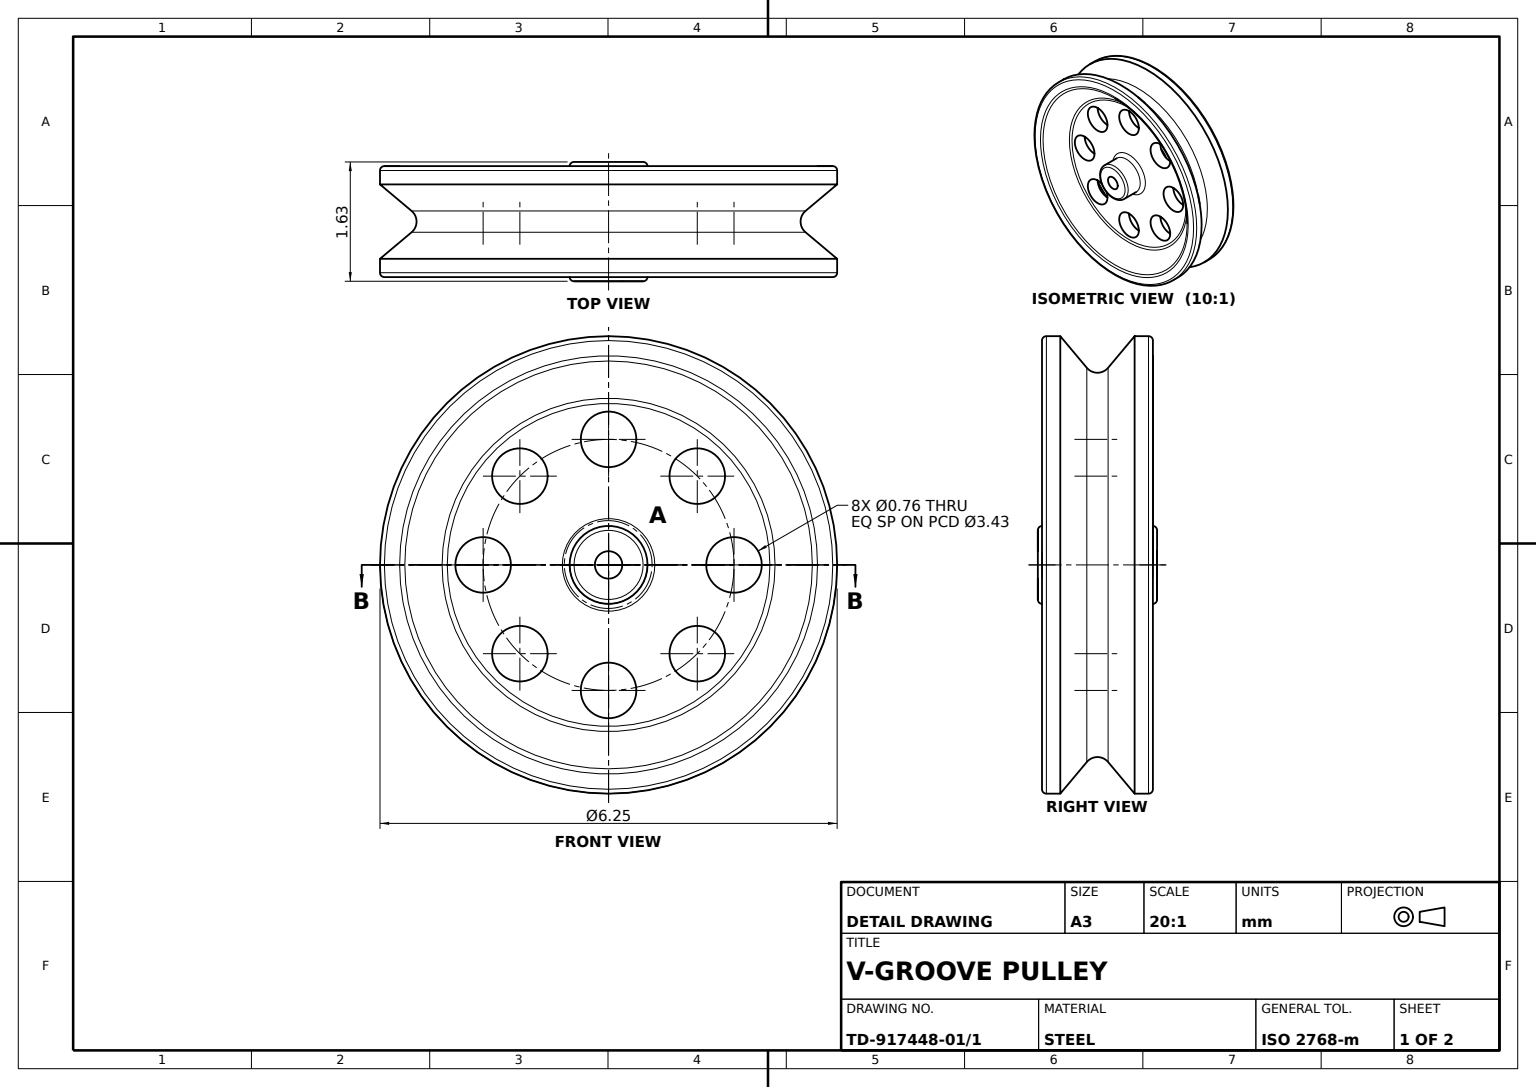
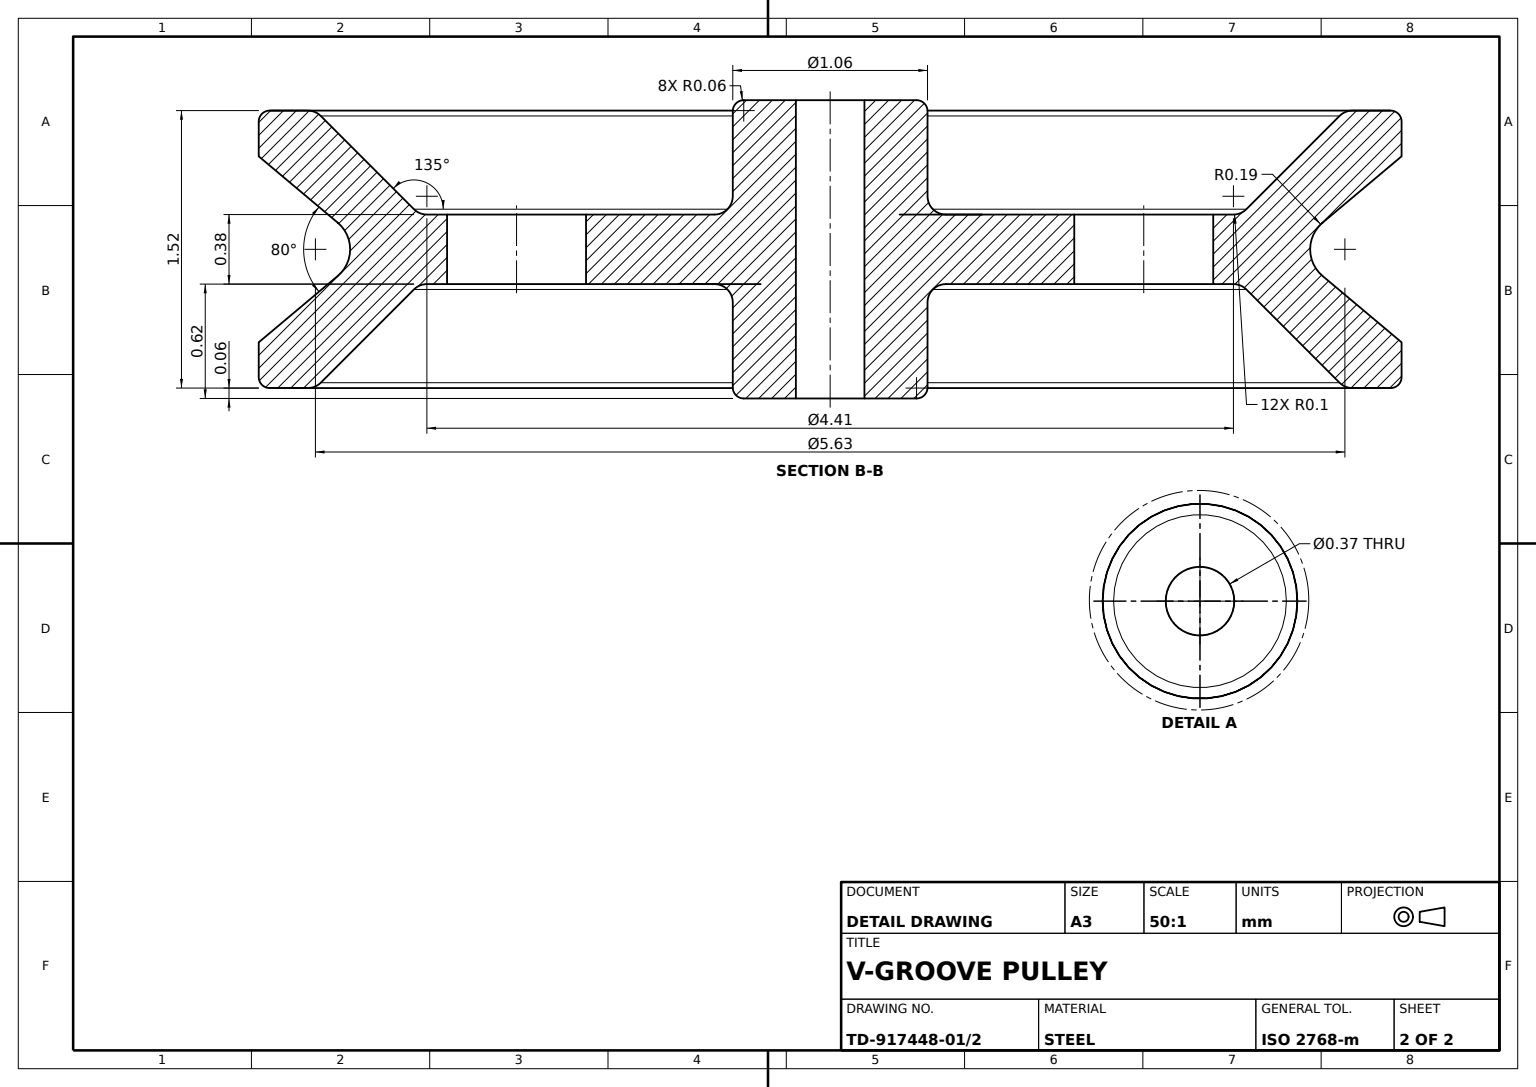
SolidWorks part; units mm, degrees
material "Plain Carbon Steel"
ref_plane "Front Plane" through (0, 0, 0) normal (0, 0, 1) x (1, 0, 0)
ref_plane "Top Plane" through (0, 0, 0) normal (0, 1, 0) x (1, 0, 0)
ref_plane "Right Plane" through (0, 0, 0) normal (1, 0, 0) x (0, 0, -1)
sketch "Pulley Profile Sketch" plane through (0, 0, 0) normal (0, 0, 1) x (1, 0, 0)
  line L0 (0, 0) -> (0, 1780.962) construction
  line L1 (0, 0) -> (1780.962, 0) construction
  line L2 (-0.815, 0.1875) -> (0.815, 0.1875)
  line L3 (0.815, 0.1875) -> (0.815, 0.5325)
  line L4 (0.815, 0.5325) -> (0.19, 0.5325)
  line L5 (0.19, 0.5325) -> (0.19, 2.2469)
  line L6 (0.19, 2.2469) -> (0.7581, 2.815)
  line L7 (0.7581, 2.815) -> (0.7581, 3.125)
  line L8 (0.7581, 3.125) -> (0.5081, 3.125)
  line L9 (0.1455, 2.6929) -> (0.5081, 3.125)
  line L10 (-0.815, 0.1875) -> (-0.815, 0.5325)
  line L11 (-0.815, 0.5325) -> (-0.19, 0.5325)
  line L12 (-0.19, 0.5325) -> (-0.19, 2.2469)
  line L13 (-0.19, 2.2469) -> (-0.7581, 2.815)
  line L14 (-0.7581, 2.815) -> (-0.7581, 3.125)
  line L15 (-0.7581, 3.125) -> (-0.5081, 3.125)
  line L16 (-0.1455, 2.6929) -> (-0.5081, 3.125)
  arc A0 (-0.1455, 2.6929) -> (0.1455, 2.6929) centre (0, 2.815) ccw
  point P17 (0, 0.1875)
  point P18 (0, 2.625)
  dimension "D8" = 0.38
  dimension "D9" = 0.19
  dimension "D6" = 135
  dimension "D1" = 0.375
  dimension "D2" = 1.065
  dimension "D3" = 3.125
  dimension "D4" = 40
  dimension "D5" = 0.25
  dimension "D7" = 2.815
  dimension "D10" = 0.815
revolve "Pulley Body Revolve" add sketch "Pulley Profile Sketch" angle 360 about L1
fillet "Edge Fillets R0.06 Set 1" radius 0.06 2 edges at (-0.7581, 0, 3.125) (0.7581, 0, 3.125)
fillet "Web Fillet R0.1" radius 0.1 6 edges at (0.19, 0, 2.2469) (-0.19, 0, 2.2469) (0.19, 0, 0.5325) (-0.19, 0, 0.5325) (-0.7581, 0, 2.815) (0.7581, 0, 2.815)
fillet "Edge Fillets R0.06 Set 2" radius 0.06 2 edges at (0.815, 0, 0.5325) (-0.815, 0, 0.5325)
sketch "Bolt Hole Sketch" plane through (-0.19, 0, 0) normal (-1, 0, 0) x (0, 0, 1)
  circle A0 centre (0, 0) radius 1.715 construction
  circle A1 centre (0, 1.715) radius 0.38
  dimension "D1" = 3.43
  dimension "D2" = 0.76
extrude "Bolt Hole Ø0.76" cut sketch "Bolt Hole Sketch" against normal through all
pattern_circular "Bolt Circle Holes 8xØ0.76" count 8 every 45 about axis through (0, 0, 0) along (1, 0, 0) of "Bolt Hole Ø0.76"
